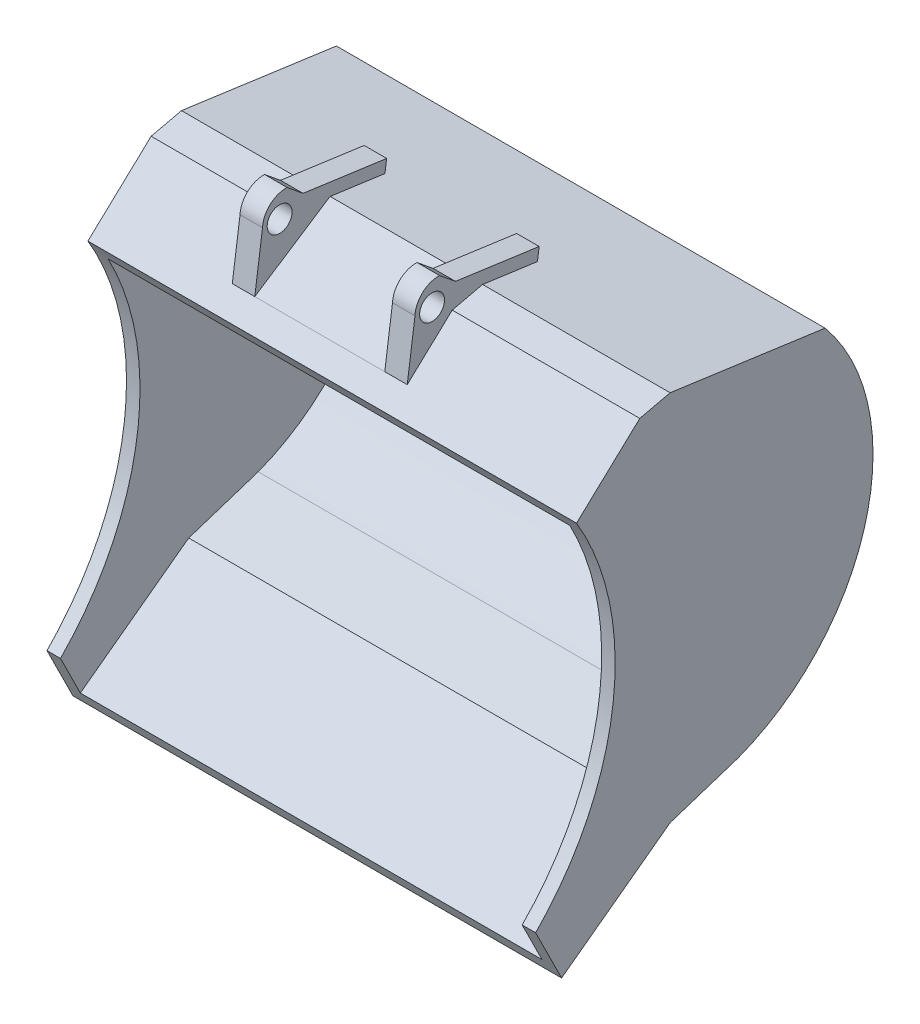
ISO-10303-21;
HEADER;
FILE_DESCRIPTION(('STEP AP214'),'2;1');
FILE_NAME('part.step','',(''),(''),'','','');
FILE_SCHEMA(('AUTOMOTIVE_DESIGN { 1 0 10303 214 1 1 1 1 }'));
ENDSEC;
DATA;
#1=APPLICATION_CONTEXT('core data for automotive mechanical design processes');
#2=APPLICATION_PROTOCOL_DEFINITION('international standard','automotive_design',2000,#1);
#3=PRODUCT_CONTEXT('',#1,'mechanical');
#4=PRODUCT('Part','Part','',(#3));
#5=PRODUCT_RELATED_PRODUCT_CATEGORY('part','',(#4));
#6=PRODUCT_DEFINITION_FORMATION('','',#4);
#7=PRODUCT_DEFINITION_CONTEXT('part definition',#1,'design');
#8=PRODUCT_DEFINITION('design','',#6,#7);
#9=PRODUCT_DEFINITION_SHAPE('','',#8);
#10=(LENGTH_UNIT() NAMED_UNIT(*) SI_UNIT(.MILLI.,.METRE.));
#11=(NAMED_UNIT(*) PLANE_ANGLE_UNIT() SI_UNIT($,.RADIAN.));
#12=(NAMED_UNIT(*) SI_UNIT($,.STERADIAN.) SOLID_ANGLE_UNIT());
#13=UNCERTAINTY_MEASURE_WITH_UNIT(LENGTH_MEASURE(1.E-05),#10,'distance_accuracy_value','');
#14=(GEOMETRIC_REPRESENTATION_CONTEXT(3) GLOBAL_UNCERTAINTY_ASSIGNED_CONTEXT((#13)) GLOBAL_UNIT_ASSIGNED_CONTEXT((#10,
#11,#12)) REPRESENTATION_CONTEXT('',''));
#15=CARTESIAN_POINT('',(0.,0.,0.));
#16=DIRECTION('',(0.,0.,1.));
#17=DIRECTION('',(1.,0.,0.));
#18=AXIS2_PLACEMENT_3D('',#15,#16,#17);
#19=CARTESIAN_POINT('',(1339.,-33.8678557689492,-244.));
#20=DIRECTION('',(0.,0.137484603920545,0.990503903922045));
#21=DIRECTION('',(0.,-0.990503903922045,0.137484603920545));
#22=AXIS2_PLACEMENT_3D('',#19,#20,#21);
#23=PLANE('',#22);
#24=DIRECTION('',(0.,0.990503903922045,-0.137484603920545));
#25=VECTOR('',#24,1.);
#26=CARTESIAN_POINT('',(1239.,-33.8678557689492,-244.));
#27=LINE('',#26,#25);
#28=CARTESIAN_POINT('',(1239.,-33.8678557689492,-244.));
#29=VERTEX_POINT('',#28);
#30=CARTESIAN_POINT('',(1239.,20.6098589467632,-251.56165321563));
#31=VERTEX_POINT('',#30);
#32=EDGE_CURVE('E476',#29,#31,#27,.T.);
#33=ORIENTED_EDGE('',*,*,#32,.T.);
#34=DIRECTION('',(-1.,0.,0.));
#35=VECTOR('',#34,1.);
#36=CARTESIAN_POINT('',(1339.,20.6098589467632,-251.56165321563));
#37=LINE('',#36,#35);
#38=CARTESIAN_POINT('',(1339.,20.6098589467632,-251.56165321563));
#39=VERTEX_POINT('',#38);
#40=EDGE_CURVE('E263',#39,#31,#37,.T.);
#41=ORIENTED_EDGE('',*,*,#40,.F.);
#42=DIRECTION('',(0.,0.990503903922045,-0.137484603920545));
#43=VECTOR('',#42,1.);
#44=CARTESIAN_POINT('',(1339.,-33.8678557689492,-244.));
#45=LINE('',#44,#43);
#46=CARTESIAN_POINT('',(1339.,-33.8678557689492,-244.));
#47=VERTEX_POINT('',#46);
#48=EDGE_CURVE('E501',#47,#39,#45,.T.);
#49=ORIENTED_EDGE('',*,*,#48,.F.);
#50=DIRECTION('',(-1.,0.,0.));
#51=VECTOR('',#50,1.);
#52=CARTESIAN_POINT('',(1339.,-33.8678557689492,-244.));
#53=LINE('',#52,#51);
#54=EDGE_CURVE('E265',#47,#29,#53,.T.);
#55=ORIENTED_EDGE('',*,*,#54,.T.);
#56=EDGE_LOOP('',(#33,#41,#49,#55));
#57=FACE_BOUND('',#56,.T.);
#58=ADVANCED_FACE('F39',(#57),#23,.F.);
#59=CARTESIAN_POINT('',(1339.,20.6098589467632,-251.56165321563));
#60=DIRECTION('',(0.,-0.990503903922045,0.137484603920544));
#61=DIRECTION('',(0.,-0.137484603920544,-0.990503903922045));
#62=AXIS2_PLACEMENT_3D('',#59,#60,#61);
#63=PLANE('',#62);
#64=DIRECTION('',(0.,0.137484603920544,0.990503903922045));
#65=VECTOR('',#64,1.);
#66=CARTESIAN_POINT('',(1239.,20.6098589467632,-251.56165321563));
#67=LINE('',#66,#65);
#68=CARTESIAN_POINT('',(1239.,72.2449516412021,120.441897980372));
#69=VERTEX_POINT('',#68);
#70=EDGE_CURVE('E485',#31,#69,#67,.T.);
#71=ORIENTED_EDGE('',*,*,#70,.T.);
#72=DIRECTION('',(-1.,0.,0.));
#73=VECTOR('',#72,1.);
#74=CARTESIAN_POINT('',(1339.,72.2449516412021,120.441897980372));
#75=LINE('',#74,#73);
#76=CARTESIAN_POINT('',(1339.,72.2449516412021,120.441897980372));
#77=VERTEX_POINT('',#76);
#78=EDGE_CURVE('E443',#77,#69,#75,.T.);
#79=ORIENTED_EDGE('',*,*,#78,.F.);
#80=DIRECTION('',(0.,0.137484603920544,0.990503903922045));
#81=VECTOR('',#80,1.);
#82=CARTESIAN_POINT('',(1339.,20.6098589467632,-251.56165321563));
#83=LINE('',#82,#81);
#84=EDGE_CURVE('E502',#39,#77,#83,.T.);
#85=ORIENTED_EDGE('',*,*,#84,.F.);
#86=ORIENTED_EDGE('',*,*,#40,.T.);
#87=EDGE_LOOP('',(#71,#79,#85,#86));
#88=FACE_BOUND('',#87,.T.);
#89=ADVANCED_FACE('F526',(#88),#63,.F.);
#90=CARTESIAN_POINT('',(1339.,72.2449516412021,120.441897980372));
#91=DIRECTION('',(0.,-0.774121532528882,0.633037007508356));
#92=DIRECTION('',(0.,-0.633037007508356,-0.774121532528882));
#93=AXIS2_PLACEMENT_3D('',#90,#91,#92);
#94=PLANE('',#93);
#95=DIRECTION('',(0.,0.633037007508356,0.774121532528882));
#96=VECTOR('',#95,1.);
#97=CARTESIAN_POINT('',(1239.,72.2449516412021,120.441897980372));
#98=LINE('',#97,#96);
#99=CARTESIAN_POINT('',(1239.,130.129855607766,191.227570914813));
#100=VERTEX_POINT('',#99);
#101=EDGE_CURVE('E484',#69,#100,#98,.T.);
#102=ORIENTED_EDGE('',*,*,#101,.T.);
#103=DIRECTION('',(-1.,0.,0.));
#104=VECTOR('',#103,1.);
#105=CARTESIAN_POINT('',(1339.,130.129855607766,191.227570914813));
#106=LINE('',#105,#104);
#107=CARTESIAN_POINT('',(1339.,130.129855607766,191.227570914813));
#108=VERTEX_POINT('',#107);
#109=EDGE_CURVE('E445',#108,#100,#106,.T.);
#110=ORIENTED_EDGE('',*,*,#109,.F.);
#111=DIRECTION('',(0.,0.633037007508356,0.774121532528882));
#112=VECTOR('',#111,1.);
#113=CARTESIAN_POINT('',(1339.,72.2449516412021,120.441897980372));
#114=LINE('',#113,#112);
#115=EDGE_CURVE('E504',#77,#108,#114,.T.);
#116=ORIENTED_EDGE('',*,*,#115,.F.);
#117=ORIENTED_EDGE('',*,*,#78,.T.);
#118=EDGE_LOOP('',(#102,#110,#116,#117));
#119=FACE_BOUND('',#118,.T.);
#120=ADVANCED_FACE('F529',(#119),#94,.F.);
#121=CARTESIAN_POINT('',(1339.,24.8813249585359,195.369514441472));
#122=DIRECTION('',(-1.,0.,0.));
#123=DIRECTION('',(0.,0.,1.));
#124=AXIS2_PLACEMENT_3D('',#121,#122,#123);
#125=CYLINDRICAL_SURFACE('',#124,105.33);
#126=CARTESIAN_POINT('',(1239.,24.8813249585359,195.369514441472));
#127=DIRECTION('',(1.,0.,0.));
#128=DIRECTION('',(0.,0.,1.));
#129=AXIS2_PLACEMENT_3D('',#126,#127,#128);
#130=CIRCLE('',#129,105.33);
#131=CARTESIAN_POINT('',(1239.,29.4466592998224,300.600529937628));
#132=VERTEX_POINT('',#131);
#133=EDGE_CURVE('E490',#100,#132,#130,.T.);
#134=ORIENTED_EDGE('',*,*,#133,.T.);
#135=DIRECTION('',(-1.,0.,0.));
#136=VECTOR('',#135,1.);
#137=CARTESIAN_POINT('',(1339.,29.4466592998224,300.600529937628));
#138=LINE('',#137,#136);
#139=CARTESIAN_POINT('',(1339.,29.4466592998224,300.600529937628));
#140=VERTEX_POINT('',#139);
#141=EDGE_CURVE('E437',#140,#132,#138,.T.);
#142=ORIENTED_EDGE('',*,*,#141,.F.);
#143=CARTESIAN_POINT('',(1339.,24.8813249585359,195.369514441472));
#144=DIRECTION('',(1.,0.,0.));
#145=DIRECTION('',(0.,0.,1.));
#146=AXIS2_PLACEMENT_3D('',#143,#144,#145);
#147=CIRCLE('',#146,105.33);
#148=EDGE_CURVE('E508',#108,#140,#147,.T.);
#149=ORIENTED_EDGE('',*,*,#148,.F.);
#150=ORIENTED_EDGE('',*,*,#109,.T.);
#151=EDGE_LOOP('',(#134,#142,#149,#150));
#152=FACE_BOUND('',#151,.T.);
#153=ADVANCED_FACE('F535',(#152),#125,.T.);
#154=CARTESIAN_POINT('',(1339.,-218.383340700178,335.));
#155=DIRECTION('',(0.,-0.137484603920545,-0.990503903922045));
#156=DIRECTION('',(0.,0.990503903922045,-0.137484603920545));
#157=AXIS2_PLACEMENT_3D('',#154,#155,#156);
#158=PLANE('',#157);
#159=DIRECTION('',(0.,-0.990503903922044,0.137484603920545));
#160=VECTOR('',#159,1.);
#161=CARTESIAN_POINT('',(1239.,-218.383340700178,335.));
#162=LINE('',#161,#160);
#163=CARTESIAN_POINT('',(1239.,-218.383340700178,335.));
#164=VERTEX_POINT('',#163);
#165=EDGE_CURVE('E489',#132,#164,#162,.T.);
#166=ORIENTED_EDGE('',*,*,#165,.T.);
#167=DIRECTION('',(-1.,0.,0.));
#168=VECTOR('',#167,1.);
#169=CARTESIAN_POINT('',(1339.,-218.383340700178,335.));
#170=LINE('',#169,#168);
#171=CARTESIAN_POINT('',(1339.,-218.383340700178,335.));
#172=VERTEX_POINT('',#171);
#173=EDGE_CURVE('E432',#172,#164,#170,.T.);
#174=ORIENTED_EDGE('',*,*,#173,.F.);
#175=DIRECTION('',(0.,-0.990503903922044,0.137484603920545));
#176=VECTOR('',#175,1.);
#177=CARTESIAN_POINT('',(1339.,-218.383340700178,335.));
#178=LINE('',#177,#176);
#179=EDGE_CURVE('E419',#140,#172,#178,.T.);
#180=ORIENTED_EDGE('',*,*,#179,.F.);
#181=ORIENTED_EDGE('',*,*,#141,.T.);
#182=EDGE_LOOP('',(#166,#174,#180,#181));
#183=FACE_BOUND('',#182,.T.);
#184=ADVANCED_FACE('F513',(#183),#158,.F.);
#185=CARTESIAN_POINT('',(1339.,24.8813249585359,224.465292997617));
#186=DIRECTION('',(-1.,0.,0.));
#187=DIRECTION('',(0.,0.,1.));
#188=AXIS2_PLACEMENT_3D('',#185,#186,#187);
#189=CYLINDRICAL_SURFACE('',#188,55.335);
#190=CARTESIAN_POINT('',(1339.,24.8813249585359,224.465292997617));
#191=DIRECTION('',(1.,0.,0.));
#192=DIRECTION('',(0.,0.,-1.));
#193=AXIS2_PLACEMENT_3D('',#190,#191,#192);
#194=CIRCLE('',#193,55.335);
#195=CARTESIAN_POINT('',(1339.,24.8813249585359,169.130292997617));
#196=VERTEX_POINT('',#195);
#197=EDGE_CURVE('E415',#196,#196,#194,.T.);
#198=ORIENTED_EDGE('',*,*,#197,.T.);
#199=EDGE_LOOP('',(#198));
#200=FACE_BOUND('',#199,.T.);
#201=CARTESIAN_POINT('',(1239.,24.8813249585359,224.465292997617));
#202=DIRECTION('',(1.,0.,0.));
#203=DIRECTION('',(0.,0.,-1.));
#204=AXIS2_PLACEMENT_3D('',#201,#202,#203);
#205=CIRCLE('',#204,55.335);
#206=CARTESIAN_POINT('',(1239.,24.8813249585359,169.130292997617));
#207=VERTEX_POINT('',#206);
#208=EDGE_CURVE('E581',#207,#207,#205,.T.);
#209=ORIENTED_EDGE('',*,*,#208,.F.);
#210=EDGE_LOOP('',(#209));
#211=FACE_BOUND('',#210,.T.);
#212=ADVANCED_FACE('F550',(#200,#211),#189,.F.);
#213=CARTESIAN_POINT('',(2173.,0.,0.));
#214=DIRECTION('',(0.,-0.990503903922045,0.137484603920545));
#215=DIRECTION('',(0.,-0.137484603920545,-0.990503903922045));
#216=AXIS2_PLACEMENT_3D('',#213,#214,#215);
#217=PLANE('',#216);
#218=DIRECTION('',(0.,-0.137484603920545,-0.990503903922045));
#219=VECTOR('',#218,1.);
#220=CARTESIAN_POINT('',(1339.,0.,0.));
#221=LINE('',#220,#219);
#222=CARTESIAN_POINT('',(1339.,0.,0.));
#223=VERTEX_POINT('',#222);
#224=EDGE_CURVE('E433',#223,#47,#221,.T.);
#225=ORIENTED_EDGE('',*,*,#224,.F.);
#226=DIRECTION('',(-1.,0.,0.));
#227=VECTOR('',#226,1.);
#228=CARTESIAN_POINT('',(2173.,0.,0.));
#229=LINE('',#228,#227);
#230=CARTESIAN_POINT('',(2173.,0.,0.));
#231=VERTEX_POINT('',#230);
#232=EDGE_CURVE('E395',#231,#223,#229,.T.);
#233=ORIENTED_EDGE('',*,*,#232,.F.);
#234=DIRECTION('',(0.,0.137484603920545,0.990503903922045));
#235=VECTOR('',#234,1.);
#236=CARTESIAN_POINT('',(2173.,0.,0.));
#237=LINE('',#236,#235);
#238=CARTESIAN_POINT('',(2173.,-95.6350517410083,-689.));
#239=VERTEX_POINT('',#238);
#240=EDGE_CURVE('E334',#239,#231,#237,.T.);
#241=ORIENTED_EDGE('',*,*,#240,.F.);
#242=DIRECTION('',(-1.,0.,0.));
#243=VECTOR('',#242,1.);
#244=CARTESIAN_POINT('',(2173.,-95.6350517410083,-689.));
#245=LINE('',#244,#243);
#246=CARTESIAN_POINT('',(0.,-95.6350517410083,-689.));
#247=VERTEX_POINT('',#246);
#248=EDGE_CURVE('E351',#239,#247,#245,.T.);
#249=ORIENTED_EDGE('',*,*,#248,.T.);
#250=DIRECTION('',(0.,0.137484603920545,0.990503903922045));
#251=VECTOR('',#250,1.);
#252=CARTESIAN_POINT('',(0.,0.,0.));
#253=LINE('',#252,#251);
#254=CARTESIAN_POINT('',(0.,0.,0.));
#255=VERTEX_POINT('',#254);
#256=EDGE_CURVE('E285',#247,#255,#253,.T.);
#257=ORIENTED_EDGE('',*,*,#256,.T.);
#258=CARTESIAN_POINT('',(561.,0.,0.));
#259=VERTEX_POINT('',#258);
#260=EDGE_CURVE('E391',#259,#255,#229,.T.);
#261=ORIENTED_EDGE('',*,*,#260,.F.);
#262=DIRECTION('',(0.,-0.137484603920545,-0.990503903922045));
#263=VECTOR('',#262,1.);
#264=CARTESIAN_POINT('',(561.,0.,0.));
#265=LINE('',#264,#263);
#266=CARTESIAN_POINT('',(561.,-33.8678557689492,-244.));
#267=VERTEX_POINT('',#266);
#268=EDGE_CURVE('E257',#259,#267,#265,.T.);
#269=ORIENTED_EDGE('',*,*,#268,.T.);
#270=CARTESIAN_POINT('',(661.,-33.8678557689492,-244.));
#271=VERTEX_POINT('',#270);
#272=EDGE_CURVE('E65',#271,#267,#53,.T.);
#273=ORIENTED_EDGE('',*,*,#272,.F.);
#274=DIRECTION('',(0.,-0.137484603920545,-0.990503903922045));
#275=VECTOR('',#274,1.);
#276=CARTESIAN_POINT('',(661.,0.,0.));
#277=LINE('',#276,#275);
#278=CARTESIAN_POINT('',(661.,0.,0.));
#279=VERTEX_POINT('',#278);
#280=EDGE_CURVE('E244',#279,#271,#277,.T.);
#281=ORIENTED_EDGE('',*,*,#280,.F.);
#282=DIRECTION('',(1.,0.,0.));
#283=VECTOR('',#282,1.);
#284=CARTESIAN_POINT('',(661.,0.,0.));
#285=LINE('',#284,#283);
#286=CARTESIAN_POINT('',(1239.,0.,0.));
#287=VERTEX_POINT('',#286);
#288=EDGE_CURVE('E493',#279,#287,#285,.T.);
#289=ORIENTED_EDGE('',*,*,#288,.T.);
#290=DIRECTION('',(0.,-0.137484603920545,-0.990503903922045));
#291=VECTOR('',#290,1.);
#292=CARTESIAN_POINT('',(1239.,0.,0.));
#293=LINE('',#292,#291);
#294=EDGE_CURVE('E474',#287,#29,#293,.T.);
#295=ORIENTED_EDGE('',*,*,#294,.T.);
#296=ORIENTED_EDGE('',*,*,#54,.F.);
#297=EDGE_LOOP('',(#225,#233,#241,#249,#257,#261,#269,#273,#281,#289,#295,#296));
#298=FACE_BOUND('',#297,.T.);
#299=ADVANCED_FACE('F41',(#298),#217,.F.);
#300=CARTESIAN_POINT('',(2173.,0.,0.));
#301=DIRECTION('',(0.,-0.974101667469916,-0.226110462898843));
#302=DIRECTION('',(0.,0.226110462898843,-0.974101667469916));
#303=AXIS2_PLACEMENT_3D('',#300,#301,#302);
#304=PLANE('',#303);
#305=DIRECTION('',(0.,0.226110462898843,-0.974101667469916));
#306=VECTOR('',#305,1.);
#307=CARTESIAN_POINT('',(1339.,0.,0.));
#308=LINE('',#307,#306);
#309=CARTESIAN_POINT('',(1339.,-31.3039778545289,134.86));
#310=VERTEX_POINT('',#309);
#311=EDGE_CURVE('E275',#310,#223,#308,.T.);
#312=ORIENTED_EDGE('',*,*,#311,.F.);
#313=DIRECTION('',(-1.,0.,0.));
#314=VECTOR('',#313,1.);
#315=CARTESIAN_POINT('',(2173.,-31.3039778545289,134.86));
#316=LINE('',#315,#314);
#317=CARTESIAN_POINT('',(2173.,-31.3039778545289,134.86));
#318=VERTEX_POINT('',#317);
#319=EDGE_CURVE('E389',#318,#310,#316,.T.);
#320=ORIENTED_EDGE('',*,*,#319,.F.);
#321=DIRECTION('',(0.,-0.226110462898843,0.974101667469916));
#322=VECTOR('',#321,1.);
#323=CARTESIAN_POINT('',(2173.,0.,0.));
#324=LINE('',#323,#322);
#325=EDGE_CURVE('E336',#231,#318,#324,.T.);
#326=ORIENTED_EDGE('',*,*,#325,.F.);
#327=ORIENTED_EDGE('',*,*,#232,.T.);
#328=EDGE_LOOP('',(#312,#320,#326,#327));
#329=FACE_BOUND('',#328,.T.);
#330=ADVANCED_FACE('F519',(#329),#304,.F.);
#331=CARTESIAN_POINT('',(2173.,-31.3039778545289,134.86));
#332=DIRECTION('',(0.,-0.730541558448307,-0.682868238666816));
#333=DIRECTION('',(0.,0.682868238666816,-0.730541558448307));
#334=AXIS2_PLACEMENT_3D('',#331,#332,#333);
#335=PLANE('',#334);
#336=DIRECTION('',(0.,0.682868238666816,-0.730541558448307));
#337=VECTOR('',#336,1.);
#338=CARTESIAN_POINT('',(1339.,-31.3039778545289,134.86));
#339=LINE('',#338,#337);
#340=EDGE_CURVE('E11',#172,#310,#339,.T.);
#341=ORIENTED_EDGE('',*,*,#340,.F.);
#342=ORIENTED_EDGE('',*,*,#173,.T.);
#343=DIRECTION('',(1.,0.,0.));
#344=VECTOR('',#343,1.);
#345=CARTESIAN_POINT('',(661.,-218.383340700178,335.));
#346=LINE('',#345,#344);
#347=CARTESIAN_POINT('',(661.,-218.383340700178,335.));
#348=VERTEX_POINT('',#347);
#349=EDGE_CURVE('E475',#348,#164,#346,.T.);
#350=ORIENTED_EDGE('',*,*,#349,.F.);
#351=CARTESIAN_POINT('',(561.,-218.383340700178,335.));
#352=VERTEX_POINT('',#351);
#353=EDGE_CURVE('E399',#348,#352,#170,.T.);
#354=ORIENTED_EDGE('',*,*,#353,.T.);
#355=DIRECTION('',(0.,0.682868238666816,-0.730541558448307));
#356=VECTOR('',#355,1.);
#357=CARTESIAN_POINT('',(561.,-31.3039778545289,134.86));
#358=LINE('',#357,#356);
#359=CARTESIAN_POINT('',(561.,-31.3039778545289,134.86));
#360=VERTEX_POINT('',#359);
#361=EDGE_CURVE('E50',#352,#360,#358,.T.);
#362=ORIENTED_EDGE('',*,*,#361,.T.);
#363=CARTESIAN_POINT('',(0.,-31.3039778545289,134.86));
#364=VERTEX_POINT('',#363);
#365=EDGE_CURVE('E390',#360,#364,#316,.T.);
#366=ORIENTED_EDGE('',*,*,#365,.T.);
#367=DIRECTION('',(0.,-0.682868238666816,0.730541558448307));
#368=VECTOR('',#367,1.);
#369=CARTESIAN_POINT('',(0.,-31.3039778545289,134.86));
#370=LINE('',#369,#368);
#371=CARTESIAN_POINT('',(0.,-294.208249741253,416.118500002598));
#372=VERTEX_POINT('',#371);
#373=EDGE_CURVE('E360',#364,#372,#370,.T.);
#374=ORIENTED_EDGE('',*,*,#373,.T.);
#375=DIRECTION('',(-1.,0.,0.));
#376=VECTOR('',#375,1.);
#377=CARTESIAN_POINT('',(2173.,-294.208249741253,416.118500002598));
#378=LINE('',#377,#376);
#379=CARTESIAN_POINT('',(2173.,-294.208249741253,416.118500002598));
#380=VERTEX_POINT('',#379);
#381=EDGE_CURVE('E383',#380,#372,#378,.T.);
#382=ORIENTED_EDGE('',*,*,#381,.F.);
#383=DIRECTION('',(0.,-0.682868238666816,0.730541558448307));
#384=VECTOR('',#383,1.);
#385=CARTESIAN_POINT('',(2173.,-31.3039778545289,134.86));
#386=LINE('',#385,#384);
#387=EDGE_CURVE('E338',#318,#380,#386,.T.);
#388=ORIENTED_EDGE('',*,*,#387,.F.);
#389=ORIENTED_EDGE('',*,*,#319,.T.);
#390=EDGE_LOOP('',(#341,#342,#350,#354,#362,#366,#374,#382,#388,#389));
#391=FACE_BOUND('',#390,.T.);
#392=ADVANCED_FACE('F400',(#391),#335,.F.);
#393=CARTESIAN_POINT('',(2173.,-919.634284323021,1469.4310249767));
#394=DIRECTION('',(-1.,0.,0.));
#395=DIRECTION('',(0.,0.,1.));
#396=AXIS2_PLACEMENT_3D('',#393,#394,#395);
#397=CYLINDRICAL_SURFACE('',#396,1225.);
#398=CARTESIAN_POINT('',(60.0000000000001,-919.634284323021,1469.4310249767));
#399=DIRECTION('',(-1.,0.,0.));
#400=DIRECTION('',(0.,0.,1.));
#401=AXIS2_PLACEMENT_3D('',#398,#399,#400);
#402=CIRCLE('',#401,1225.);
#403=CARTESIAN_POINT('',(60.,-348.114078031214,385.922993718895));
#404=VERTEX_POINT('',#403);
#405=CARTESIAN_POINT('',(60.0000000000001,-1780.60824974125,598.02478740894));
#406=VERTEX_POINT('',#405);
#407=EDGE_CURVE('E305',#404,#406,#402,.T.);
#408=ORIENTED_EDGE('',*,*,#407,.F.);
#409=DIRECTION('',(-1.,0.,0.));
#410=VECTOR('',#409,1.);
#411=CARTESIAN_POINT('',(2113.,-348.114078031214,385.922993718895));
#412=LINE('',#411,#410);
#413=CARTESIAN_POINT('',(2113.,-348.114078031214,385.922993718895));
#414=VERTEX_POINT('',#413);
#415=EDGE_CURVE('E297',#414,#404,#412,.T.);
#416=ORIENTED_EDGE('',*,*,#415,.F.);
#417=CARTESIAN_POINT('',(2113.,-919.634284323021,1469.4310249767));
#418=DIRECTION('',(-1.,0.,0.));
#419=DIRECTION('',(0.,0.,1.));
#420=AXIS2_PLACEMENT_3D('',#417,#418,#419);
#421=CIRCLE('',#420,1225.);
#422=CARTESIAN_POINT('',(2113.,-1780.60824974125,598.02478740894));
#423=VERTEX_POINT('',#422);
#424=EDGE_CURVE('E302',#414,#423,#421,.T.);
#425=ORIENTED_EDGE('',*,*,#424,.T.);
#426=DIRECTION('',(-1.,0.,0.));
#427=VECTOR('',#426,1.);
#428=CARTESIAN_POINT('',(2173.,-1780.60824974125,598.02478740894));
#429=LINE('',#428,#427);
#430=CARTESIAN_POINT('',(2173.,-1780.60824974125,598.02478740894));
#431=VERTEX_POINT('',#430);
#432=EDGE_CURVE('E381',#431,#423,#429,.T.);
#433=ORIENTED_EDGE('',*,*,#432,.F.);
#434=CARTESIAN_POINT('',(2173.,-919.634284323021,1469.4310249767));
#435=DIRECTION('',(-1.,0.,0.));
#436=DIRECTION('',(0.,0.,1.));
#437=AXIS2_PLACEMENT_3D('',#434,#435,#436);
#438=CIRCLE('',#437,1225.);
#439=EDGE_CURVE('E343',#380,#431,#438,.T.);
#440=ORIENTED_EDGE('',*,*,#439,.F.);
#441=ORIENTED_EDGE('',*,*,#381,.T.);
#442=CARTESIAN_POINT('',(0.,-919.634284323021,1469.4310249767));
#443=DIRECTION('',(-1.,0.,0.));
#444=DIRECTION('',(0.,0.,1.));
#445=AXIS2_PLACEMENT_3D('',#442,#443,#444);
#446=CIRCLE('',#445,1225.);
#447=CARTESIAN_POINT('',(0.,-1780.60824974125,598.02478740894));
#448=VERTEX_POINT('',#447);
#449=EDGE_CURVE('E357',#372,#448,#446,.T.);
#450=ORIENTED_EDGE('',*,*,#449,.T.);
#451=EDGE_CURVE('E379',#406,#448,#429,.T.);
#452=ORIENTED_EDGE('',*,*,#451,.F.);
#453=EDGE_LOOP('',(#408,#416,#425,#433,#440,#441,#450,#452));
#454=FACE_BOUND('',#453,.T.);
#455=ADVANCED_FACE('F605',(#454),#397,.F.);
#456=CARTESIAN_POINT('',(2173.,-2012.60824974125,482.525187131697));
#457=DIRECTION('',(0.,0.445668249515807,-0.895198196699209));
#458=DIRECTION('',(0.,0.895198196699209,0.445668249515807));
#459=AXIS2_PLACEMENT_3D('',#456,#457,#458);
#460=PLANE('',#459);
#461=DIRECTION('',(0.,-0.895198196699209,-0.445668249515807));
#462=VECTOR('',#461,1.);
#463=CARTESIAN_POINT('',(60.,-1132.73844899319,920.562300417985));
#464=LINE('',#463,#462);
#465=CARTESIAN_POINT('',(60.,-1958.06776543082,509.67779116955));
#466=VERTEX_POINT('',#465);
#467=EDGE_CURVE('E314',#406,#466,#464,.T.);
#468=ORIENTED_EDGE('',*,*,#467,.F.);
#469=ORIENTED_EDGE('',*,*,#451,.T.);
#470=DIRECTION('',(0.,-0.895198196699209,-0.445668249515807));
#471=VECTOR('',#470,1.);
#472=CARTESIAN_POINT('',(0.,-2012.60824974125,482.525187131697));
#473=LINE('',#472,#471);
#474=CARTESIAN_POINT('',(0.,-2012.60824974125,482.525187131697));
#475=VERTEX_POINT('',#474);
#476=EDGE_CURVE('E362',#448,#475,#473,.T.);
#477=ORIENTED_EDGE('',*,*,#476,.T.);
#478=DIRECTION('',(-1.,0.,0.));
#479=VECTOR('',#478,1.);
#480=CARTESIAN_POINT('',(2173.,-2012.60824974125,482.525187131697));
#481=LINE('',#480,#479);
#482=CARTESIAN_POINT('',(2173.,-2012.60824974125,482.525187131697));
#483=VERTEX_POINT('',#482);
#484=EDGE_CURVE('E380',#483,#475,#481,.T.);
#485=ORIENTED_EDGE('',*,*,#484,.F.);
#486=DIRECTION('',(0.,-0.895198196699209,-0.445668249515807));
#487=VECTOR('',#486,1.);
#488=CARTESIAN_POINT('',(2173.,-2012.60824974125,482.525187131697));
#489=LINE('',#488,#487);
#490=EDGE_CURVE('E341',#431,#483,#489,.T.);
#491=ORIENTED_EDGE('',*,*,#490,.F.);
#492=ORIENTED_EDGE('',*,*,#432,.T.);
#493=DIRECTION('',(0.,-0.895198196699209,-0.445668249515807));
#494=VECTOR('',#493,1.);
#495=CARTESIAN_POINT('',(2113.,-1132.73844899319,920.562300417985));
#496=LINE('',#495,#494);
#497=CARTESIAN_POINT('',(2113.,-1958.06776543082,509.67779116955));
#498=VERTEX_POINT('',#497);
#499=EDGE_CURVE('E306',#423,#498,#496,.T.);
#500=ORIENTED_EDGE('',*,*,#499,.T.);
#501=DIRECTION('',(-1.,0.,0.));
#502=VECTOR('',#501,1.);
#503=CARTESIAN_POINT('',(2173.,-1958.06776543082,509.67779116955));
#504=LINE('',#503,#502);
#505=EDGE_CURVE('E318',#498,#466,#504,.T.);
#506=ORIENTED_EDGE('',*,*,#505,.T.);
#507=EDGE_LOOP('',(#468,#469,#477,#485,#491,#492,#500,#506));
#508=FACE_BOUND('',#507,.T.);
#509=ADVANCED_FACE('F604',(#508),#460,.F.);
#510=ORIENTED_EDGE('',*,*,#365,.F.);
#511=DIRECTION('',(0.,0.226110462898843,-0.974101667469916));
#512=VECTOR('',#511,1.);
#513=CARTESIAN_POINT('',(561.,0.,0.));
#514=LINE('',#513,#512);
#515=EDGE_CURVE('E266',#360,#259,#514,.T.);
#516=ORIENTED_EDGE('',*,*,#515,.T.);
#517=ORIENTED_EDGE('',*,*,#260,.T.);
#518=DIRECTION('',(0.,-0.226110462898843,0.974101667469916));
#519=VECTOR('',#518,1.);
#520=CARTESIAN_POINT('',(0.,0.,0.));
#521=LINE('',#520,#519);
#522=EDGE_CURVE('E353',#255,#364,#521,.T.);
#523=ORIENTED_EDGE('',*,*,#522,.T.);
#524=EDGE_LOOP('',(#510,#516,#517,#523));
#525=FACE_BOUND('',#524,.T.);
#526=ADVANCED_FACE('F406',(#525),#304,.F.);
#527=CARTESIAN_POINT('',(2173.,-1656.,-2.02801509938802E-13));
#528=DIRECTION('',(0.,0.804208645219496,0.59434708290209));
#529=DIRECTION('',(0.,-0.59434708290209,0.804208645219496));
#530=AXIS2_PLACEMENT_3D('',#527,#528,#529);
#531=PLANE('',#530);
#532=DIRECTION('',(0.,0.59434708290209,-0.804208645219496));
#533=VECTOR('',#532,1.);
#534=CARTESIAN_POINT('',(0.,-1656.,-2.02801509938802E-13));
#535=LINE('',#534,#533);
#536=CARTESIAN_POINT('',(0.,-1656.,-2.02801509938802E-13));
#537=VERTEX_POINT('',#536);
#538=EDGE_CURVE('E365',#475,#537,#535,.T.);
#539=ORIENTED_EDGE('',*,*,#538,.T.);
#540=DIRECTION('',(-1.,0.,0.));
#541=VECTOR('',#540,1.);
#542=CARTESIAN_POINT('',(2173.,-1656.,-2.02801509938802E-13));
#543=LINE('',#542,#541);
#544=CARTESIAN_POINT('',(2173.,-1656.,-2.02801509938802E-13));
#545=VERTEX_POINT('',#544);
#546=EDGE_CURVE('E372',#545,#537,#543,.T.);
#547=ORIENTED_EDGE('',*,*,#546,.F.);
#548=DIRECTION('',(0.,0.59434708290209,-0.804208645219496));
#549=VECTOR('',#548,1.);
#550=CARTESIAN_POINT('',(2173.,-1656.,-2.02801509938802E-13));
#551=LINE('',#550,#549);
#552=EDGE_CURVE('E344',#483,#545,#551,.T.);
#553=ORIENTED_EDGE('',*,*,#552,.F.);
#554=ORIENTED_EDGE('',*,*,#484,.T.);
#555=EDGE_LOOP('',(#539,#547,#553,#554));
#556=FACE_BOUND('',#555,.T.);
#557=ADVANCED_FACE('F603',(#556),#531,.F.);
#558=CARTESIAN_POINT('',(2173.,-1656.,-2.02801509938802E-13));
#559=DIRECTION('',(0.,0.951056516295152,0.309016994374952));
#560=DIRECTION('',(0.,-0.309016994374952,0.951056516295152));
#561=AXIS2_PLACEMENT_3D('',#558,#559,#560);
#562=PLANE('',#561);
#563=DIRECTION('',(0.,0.309016994374952,-0.951056516295152));
#564=VECTOR('',#563,1.);
#565=CARTESIAN_POINT('',(0.,-1656.,-2.02801509938802E-13));
#566=LINE('',#565,#564);
#567=CARTESIAN_POINT('',(0.,-1558.12025642121,-301.242875435373));
#568=VERTEX_POINT('',#567);
#569=EDGE_CURVE('E368',#537,#568,#566,.T.);
#570=ORIENTED_EDGE('',*,*,#569,.T.);
#571=DIRECTION('',(-1.,0.,0.));
#572=VECTOR('',#571,1.);
#573=CARTESIAN_POINT('',(2173.,-1558.12025642121,-301.242875435373));
#574=LINE('',#573,#572);
#575=CARTESIAN_POINT('',(2173.,-1558.12025642121,-301.242875435373));
#576=VERTEX_POINT('',#575);
#577=EDGE_CURVE('E371',#576,#568,#574,.T.);
#578=ORIENTED_EDGE('',*,*,#577,.F.);
#579=DIRECTION('',(0.,0.309016994374952,-0.951056516295152));
#580=VECTOR('',#579,1.);
#581=CARTESIAN_POINT('',(2173.,-1656.,-2.02801509938802E-13));
#582=LINE('',#581,#580);
#583=EDGE_CURVE('E350',#545,#576,#582,.T.);
#584=ORIENTED_EDGE('',*,*,#583,.F.);
#585=ORIENTED_EDGE('',*,*,#546,.T.);
#586=EDGE_LOOP('',(#570,#578,#584,#585));
#587=FACE_BOUND('',#586,.T.);
#588=ADVANCED_FACE('F606',(#587),#562,.F.);
#589=CARTESIAN_POINT('',(2173.,-688.25,27.7339276886459));
#590=DIRECTION('',(-1.,0.,0.));
#591=DIRECTION('',(0.,0.,1.));
#592=AXIS2_PLACEMENT_3D('',#589,#590,#591);
#593=CYLINDRICAL_SURFACE('',#592,930.);
#594=CARTESIAN_POINT('',(0.,-688.25,27.7339276886459));
#595=DIRECTION('',(1.,0.,0.));
#596=DIRECTION('',(0.,0.,1.));
#597=AXIS2_PLACEMENT_3D('',#594,#595,#596);
#598=CIRCLE('',#597,930.);
#599=EDGE_CURVE('E340',#568,#247,#598,.T.);
#600=ORIENTED_EDGE('',*,*,#599,.T.);
#601=ORIENTED_EDGE('',*,*,#248,.F.);
#602=CARTESIAN_POINT('',(2173.,-688.25,27.7339276886459));
#603=DIRECTION('',(1.,0.,0.));
#604=DIRECTION('',(0.,0.,1.));
#605=AXIS2_PLACEMENT_3D('',#602,#603,#604);
#606=CIRCLE('',#605,930.);
#607=EDGE_CURVE('E349',#576,#239,#606,.T.);
#608=ORIENTED_EDGE('',*,*,#607,.F.);
#609=ORIENTED_EDGE('',*,*,#577,.T.);
#610=EDGE_LOOP('',(#600,#601,#608,#609));
#611=FACE_BOUND('',#610,.T.);
#612=ADVANCED_FACE('F623',(#611),#593,.T.);
#613=CARTESIAN_POINT('',(2173.,-688.25,27.7339276886459));
#614=DIRECTION('',(-1.,0.,0.));
#615=DIRECTION('',(0.,0.,1.));
#616=AXIS2_PLACEMENT_3D('',#613,#614,#615);
#617=PLANE('',#616);
#618=ORIENTED_EDGE('',*,*,#240,.T.);
#619=ORIENTED_EDGE('',*,*,#325,.T.);
#620=ORIENTED_EDGE('',*,*,#387,.T.);
#621=ORIENTED_EDGE('',*,*,#439,.T.);
#622=ORIENTED_EDGE('',*,*,#490,.T.);
#623=ORIENTED_EDGE('',*,*,#552,.T.);
#624=ORIENTED_EDGE('',*,*,#583,.T.);
#625=ORIENTED_EDGE('',*,*,#607,.T.);
#626=EDGE_LOOP('',(#618,#619,#620,#621,#622,#623,#624,#625));
#627=FACE_BOUND('',#626,.T.);
#628=ADVANCED_FACE('F628',(#627),#617,.F.);
#629=CARTESIAN_POINT('',(0.,-688.25,27.7339276886459));
#630=DIRECTION('',(-1.,0.,0.));
#631=DIRECTION('',(0.,0.,1.));
#632=AXIS2_PLACEMENT_3D('',#629,#630,#631);
#633=PLANE('',#632);
#634=ORIENTED_EDGE('',*,*,#256,.F.);
#635=ORIENTED_EDGE('',*,*,#599,.F.);
#636=ORIENTED_EDGE('',*,*,#569,.F.);
#637=ORIENTED_EDGE('',*,*,#538,.F.);
#638=ORIENTED_EDGE('',*,*,#476,.F.);
#639=ORIENTED_EDGE('',*,*,#449,.F.);
#640=ORIENTED_EDGE('',*,*,#373,.F.);
#641=ORIENTED_EDGE('',*,*,#522,.F.);
#642=EDGE_LOOP('',(#634,#635,#636,#637,#638,#639,#640,#641));
#643=FACE_BOUND('',#642,.T.);
#644=ADVANCED_FACE('F633',(#643),#633,.T.);
#645=CARTESIAN_POINT('',(2173.,-59.4302342353227,8.24907623523268));
#646=DIRECTION('',(0.,-0.990503903922045,0.137484603920545));
#647=DIRECTION('',(0.,-0.137484603920545,-0.990503903922045));
#648=AXIS2_PLACEMENT_3D('',#645,#646,#647);
#649=PLANE('',#648);
#650=DIRECTION('',(0.,0.137484603920545,0.990503903922045));
#651=VECTOR('',#650,1.);
#652=CARTESIAN_POINT('',(60.,-68.6627674018115,-58.2664453847878));
#653=LINE('',#652,#651);
#654=CARTESIAN_POINT('',(60.,-151.794421903552,-657.186076931753));
#655=VERTEX_POINT('',#654);
#656=CARTESIAN_POINT('',(60.,-60.9569139254462,-2.74984400735522));
#657=VERTEX_POINT('',#656);
#658=EDGE_CURVE('E274',#655,#657,#653,.T.);
#659=ORIENTED_EDGE('',*,*,#658,.F.);
#660=DIRECTION('',(-1.,0.,0.));
#661=VECTOR('',#660,1.);
#662=CARTESIAN_POINT('',(2113.,-151.794421903552,-657.186076931753));
#663=LINE('',#662,#661);
#664=CARTESIAN_POINT('',(2113.,-151.794421903552,-657.186076931753));
#665=VERTEX_POINT('',#664);
#666=EDGE_CURVE('E287',#665,#655,#663,.T.);
#667=ORIENTED_EDGE('',*,*,#666,.F.);
#668=DIRECTION('',(0.,0.137484603920545,0.990503903922045));
#669=VECTOR('',#668,1.);
#670=CARTESIAN_POINT('',(2113.,-68.6627674018115,-58.2664453847878));
#671=LINE('',#670,#669);
#672=CARTESIAN_POINT('',(2113.,-60.9569139254462,-2.74984400735522));
#673=VERTEX_POINT('',#672);
#674=EDGE_CURVE('E283',#665,#673,#671,.T.);
#675=ORIENTED_EDGE('',*,*,#674,.T.);
#676=DIRECTION('',(-1.,0.,0.));
#677=VECTOR('',#676,1.);
#678=CARTESIAN_POINT('',(2173.,-60.9569139254462,-2.74984400735522));
#679=LINE('',#678,#677);
#680=EDGE_CURVE('E276',#673,#657,#679,.T.);
#681=ORIENTED_EDGE('',*,*,#680,.T.);
#682=EDGE_LOOP('',(#659,#667,#675,#681));
#683=FACE_BOUND('',#682,.T.);
#684=ADVANCED_FACE('F632',(#683),#649,.T.);
#685=CARTESIAN_POINT('',(2173.,-58.446100048195,-13.5666277739306));
#686=DIRECTION('',(0.,-0.974101667469916,-0.226110462898843));
#687=DIRECTION('',(0.,0.226110462898843,-0.974101667469916));
#688=AXIS2_PLACEMENT_3D('',#685,#686,#687);
#689=PLANE('',#688);
#690=DIRECTION('',(0.,-0.226110462898843,0.974101667469916));
#691=VECTOR('',#690,1.);
#692=CARTESIAN_POINT('',(60.,-99.7420538044702,164.339590708957));
#693=LINE('',#692,#691);
#694=CARTESIAN_POINT('',(60.,-86.1149109466855,105.632786917407));
#695=VERTEX_POINT('',#694);
#696=EDGE_CURVE('E279',#657,#695,#693,.T.);
#697=ORIENTED_EDGE('',*,*,#696,.F.);
#698=ORIENTED_EDGE('',*,*,#680,.F.);
#699=DIRECTION('',(0.,-0.226110462898843,0.974101667469916));
#700=VECTOR('',#699,1.);
#701=CARTESIAN_POINT('',(2113.,-99.7420538044702,164.339590708957));
#702=LINE('',#701,#700);
#703=CARTESIAN_POINT('',(2113.,-86.1149109466855,105.632786917407));
#704=VERTEX_POINT('',#703);
#705=EDGE_CURVE('E290',#673,#704,#702,.T.);
#706=ORIENTED_EDGE('',*,*,#705,.T.);
#707=DIRECTION('',(-1.,0.,0.));
#708=VECTOR('',#707,1.);
#709=CARTESIAN_POINT('',(2173.,-86.1149109466855,105.632786917407));
#710=LINE('',#709,#708);
#711=EDGE_CURVE('E282',#704,#695,#710,.T.);
#712=ORIENTED_EDGE('',*,*,#711,.T.);
#713=EDGE_LOOP('',(#697,#698,#706,#712));
#714=FACE_BOUND('',#713,.T.);
#715=ADVANCED_FACE('F659',(#714),#689,.T.);
#716=CARTESIAN_POINT('',(2173.,-75.1364713614273,93.8879056799911));
#717=DIRECTION('',(0.,-0.730541558448307,-0.682868238666816));
#718=DIRECTION('',(0.,0.682868238666816,-0.730541558448307));
#719=AXIS2_PLACEMENT_3D('',#716,#717,#718);
#720=PLANE('',#719);
#721=DIRECTION('',(0.,-0.682868238666816,0.730541558448307));
#722=VECTOR('',#721,1.);
#723=CARTESIAN_POINT('',(60.,-328.035033606346,364.442163925238));
#724=LINE('',#723,#722);
#725=EDGE_CURVE('E293',#695,#404,#724,.T.);
#726=ORIENTED_EDGE('',*,*,#725,.F.);
#727=ORIENTED_EDGE('',*,*,#711,.F.);
#728=DIRECTION('',(0.,-0.682868238666816,0.730541558448307));
#729=VECTOR('',#728,1.);
#730=CARTESIAN_POINT('',(2113.,-328.035033606346,364.442163925238));
#731=LINE('',#730,#729);
#732=EDGE_CURVE('E299',#704,#414,#731,.T.);
#733=ORIENTED_EDGE('',*,*,#732,.T.);
#734=ORIENTED_EDGE('',*,*,#415,.T.);
#735=EDGE_LOOP('',(#726,#727,#733,#734));
#736=FACE_BOUND('',#735,.T.);
#737=ADVANCED_FACE('F656',(#736),#720,.T.);
#738=CARTESIAN_POINT('',(2173.,-1607.74748128683,35.6608249741252));
#739=DIRECTION('',(0.,0.804208645219496,0.59434708290209));
#740=DIRECTION('',(0.,-0.59434708290209,0.804208645219496));
#741=AXIS2_PLACEMENT_3D('',#738,#739,#740);
#742=PLANE('',#741);
#743=DIRECTION('',(0.,0.59434708290209,-0.804208645219496));
#744=VECTOR('',#743,1.);
#745=CARTESIAN_POINT('',(60.,-1279.14752575625,-408.966452013734));
#746=LINE('',#745,#744);
#747=CARTESIAN_POINT('',(60.,-1601.95057574235,27.8170554184155));
#748=VERTEX_POINT('',#747);
#749=EDGE_CURVE('E313',#466,#748,#746,.T.);
#750=ORIENTED_EDGE('',*,*,#749,.F.);
#751=ORIENTED_EDGE('',*,*,#505,.F.);
#752=DIRECTION('',(0.,0.59434708290209,-0.804208645219496));
#753=VECTOR('',#752,1.);
#754=CARTESIAN_POINT('',(2113.,-1279.14752575625,-408.966452013734));
#755=LINE('',#754,#753);
#756=CARTESIAN_POINT('',(2113.,-1601.95057574235,27.8170554184155));
#757=VERTEX_POINT('',#756);
#758=EDGE_CURVE('E304',#498,#757,#755,.T.);
#759=ORIENTED_EDGE('',*,*,#758,.T.);
#760=DIRECTION('',(-1.,0.,0.));
#761=VECTOR('',#760,1.);
#762=CARTESIAN_POINT('',(2173.,-1601.95057574235,27.8170554184155));
#763=LINE('',#762,#761);
#764=EDGE_CURVE('E312',#757,#748,#763,.T.);
#765=ORIENTED_EDGE('',*,*,#764,.T.);
#766=EDGE_LOOP('',(#750,#751,#759,#765));
#767=FACE_BOUND('',#766,.T.);
#768=ADVANCED_FACE('F655',(#767),#742,.T.);
#769=CARTESIAN_POINT('',(2173.,-1598.93660902229,18.5410196624969));
#770=DIRECTION('',(0.,0.951056516295152,0.309016994374952));
#771=DIRECTION('',(0.,-0.309016994374952,0.951056516295152));
#772=AXIS2_PLACEMENT_3D('',#769,#770,#771);
#773=PLANE('',#772);
#774=DIRECTION('',(0.,0.309016994374952,-0.951056516295152));
#775=VECTOR('',#774,1.);
#776=CARTESIAN_POINT('',(60.,-1514.67550401723,-240.787996035764));
#777=LINE('',#776,#775);
#778=CARTESIAN_POINT('',(60.,-1501.50375553248,-281.326469503095));
#779=VERTEX_POINT('',#778);
#780=EDGE_CURVE('E311',#748,#779,#777,.T.);
#781=ORIENTED_EDGE('',*,*,#780,.F.);
#782=ORIENTED_EDGE('',*,*,#764,.F.);
#783=DIRECTION('',(0.,0.309016994374952,-0.951056516295152));
#784=VECTOR('',#783,1.);
#785=CARTESIAN_POINT('',(2113.,-1514.67550401723,-240.787996035764));
#786=LINE('',#785,#784);
#787=CARTESIAN_POINT('',(2113.,-1501.50375553248,-281.326469503095));
#788=VERTEX_POINT('',#787);
#789=EDGE_CURVE('E307',#757,#788,#786,.T.);
#790=ORIENTED_EDGE('',*,*,#789,.T.);
#791=DIRECTION('',(-1.,0.,0.));
#792=VECTOR('',#791,1.);
#793=CARTESIAN_POINT('',(2113.,-1501.50375553248,-281.326469503095));
#794=LINE('',#793,#792);
#795=EDGE_CURVE('E295',#788,#779,#794,.T.);
#796=ORIENTED_EDGE('',*,*,#795,.T.);
#797=EDGE_LOOP('',(#781,#782,#790,#796));
#798=FACE_BOUND('',#797,.T.);
#799=ADVANCED_FACE('F648',(#798),#773,.T.);
#800=CARTESIAN_POINT('',(2173.,-688.25,27.7339276886459));
#801=DIRECTION('',(-1.,0.,0.));
#802=DIRECTION('',(0.,0.,1.));
#803=AXIS2_PLACEMENT_3D('',#800,#801,#802);
#804=CYLINDRICAL_SURFACE('',#803,870.);
#805=CARTESIAN_POINT('',(60.0000000000001,-688.25,27.7339276886459));
#806=DIRECTION('',(-1.,0.,0.));
#807=DIRECTION('',(0.,0.,1.));
#808=AXIS2_PLACEMENT_3D('',#805,#806,#807);
#809=CIRCLE('',#808,870.);
#810=EDGE_CURVE('E286',#779,#655,#809,.F.);
#811=ORIENTED_EDGE('',*,*,#810,.F.);
#812=ORIENTED_EDGE('',*,*,#795,.F.);
#813=CARTESIAN_POINT('',(2113.,-688.25,27.7339276886459));
#814=DIRECTION('',(-1.,0.,0.));
#815=DIRECTION('',(0.,0.,1.));
#816=AXIS2_PLACEMENT_3D('',#813,#814,#815);
#817=CIRCLE('',#816,870.);
#818=EDGE_CURVE('E291',#788,#665,#817,.F.);
#819=ORIENTED_EDGE('',*,*,#818,.T.);
#820=ORIENTED_EDGE('',*,*,#666,.T.);
#821=EDGE_LOOP('',(#811,#812,#819,#820));
#822=FACE_BOUND('',#821,.T.);
#823=ADVANCED_FACE('F644',(#822),#804,.F.);
#824=CARTESIAN_POINT('',(2113.,-688.25,27.7339276886459));
#825=DIRECTION('',(-1.,0.,0.));
#826=DIRECTION('',(0.,0.,1.));
#827=AXIS2_PLACEMENT_3D('',#824,#825,#826);
#828=PLANE('',#827);
#829=ORIENTED_EDGE('',*,*,#674,.F.);
#830=ORIENTED_EDGE('',*,*,#818,.F.);
#831=ORIENTED_EDGE('',*,*,#789,.F.);
#832=ORIENTED_EDGE('',*,*,#758,.F.);
#833=ORIENTED_EDGE('',*,*,#499,.F.);
#834=ORIENTED_EDGE('',*,*,#424,.F.);
#835=ORIENTED_EDGE('',*,*,#732,.F.);
#836=ORIENTED_EDGE('',*,*,#705,.F.);
#837=EDGE_LOOP('',(#829,#830,#831,#832,#833,#834,#835,#836));
#838=FACE_BOUND('',#837,.T.);
#839=ADVANCED_FACE('F639',(#838),#828,.T.);
#840=CARTESIAN_POINT('',(60.,-688.25,27.7339276886459));
#841=DIRECTION('',(-1.,0.,0.));
#842=DIRECTION('',(0.,0.,1.));
#843=AXIS2_PLACEMENT_3D('',#840,#841,#842);
#844=PLANE('',#843);
#845=ORIENTED_EDGE('',*,*,#658,.T.);
#846=ORIENTED_EDGE('',*,*,#696,.T.);
#847=ORIENTED_EDGE('',*,*,#725,.T.);
#848=ORIENTED_EDGE('',*,*,#407,.T.);
#849=ORIENTED_EDGE('',*,*,#467,.T.);
#850=ORIENTED_EDGE('',*,*,#749,.T.);
#851=ORIENTED_EDGE('',*,*,#780,.T.);
#852=ORIENTED_EDGE('',*,*,#810,.T.);
#853=EDGE_LOOP('',(#845,#846,#847,#848,#849,#850,#851,#852));
#854=FACE_BOUND('',#853,.T.);
#855=ADVANCED_FACE('F566',(#854),#844,.F.);
#856=CARTESIAN_POINT('',(1339.,24.8813249585359,195.369514441472));
#857=DIRECTION('',(-1.,0.,0.));
#858=DIRECTION('',(0.,0.,1.));
#859=AXIS2_PLACEMENT_3D('',#856,#857,#858);
#860=PLANE('',#859);
#861=ORIENTED_EDGE('',*,*,#197,.F.);
#862=EDGE_LOOP('',(#861));
#863=FACE_BOUND('',#862,.T.);
#864=ORIENTED_EDGE('',*,*,#340,.T.);
#865=ORIENTED_EDGE('',*,*,#311,.T.);
#866=ORIENTED_EDGE('',*,*,#224,.T.);
#867=ORIENTED_EDGE('',*,*,#48,.T.);
#868=ORIENTED_EDGE('',*,*,#84,.T.);
#869=ORIENTED_EDGE('',*,*,#115,.T.);
#870=ORIENTED_EDGE('',*,*,#148,.T.);
#871=ORIENTED_EDGE('',*,*,#179,.T.);
#872=EDGE_LOOP('',(#864,#865,#866,#867,#868,#869,#870,#871));
#873=FACE_BOUND('',#872,.T.);
#874=ADVANCED_FACE('F511',(#863,#873),#860,.F.);
#875=CARTESIAN_POINT('',(561.,24.8813249585359,195.369514441472));
#876=DIRECTION('',(-1.,0.,0.));
#877=DIRECTION('',(0.,0.,1.));
#878=AXIS2_PLACEMENT_3D('',#875,#876,#877);
#879=PLANE('',#878);
#880=CARTESIAN_POINT('',(561.,24.8813249585359,224.465292997617));
#881=DIRECTION('',(1.,0.,0.));
#882=DIRECTION('',(0.,0.,-1.));
#883=AXIS2_PLACEMENT_3D('',#880,#881,#882);
#884=CIRCLE('',#883,55.335);
#885=CARTESIAN_POINT('',(561.,24.8813249585359,169.130292997617));
#886=VERTEX_POINT('',#885);
#887=EDGE_CURVE('E417',#886,#886,#884,.T.);
#888=ORIENTED_EDGE('',*,*,#887,.T.);
#889=EDGE_LOOP('',(#888));
#890=FACE_BOUND('',#889,.T.);
#891=ORIENTED_EDGE('',*,*,#515,.F.);
#892=ORIENTED_EDGE('',*,*,#361,.F.);
#893=DIRECTION('',(0.,-0.990503903922044,0.137484603920545));
#894=VECTOR('',#893,1.);
#895=CARTESIAN_POINT('',(561.,-218.383340700178,335.));
#896=LINE('',#895,#894);
#897=CARTESIAN_POINT('',(561.,29.4466592998224,300.600529937628));
#898=VERTEX_POINT('',#897);
#899=EDGE_CURVE('E431',#898,#352,#896,.T.);
#900=ORIENTED_EDGE('',*,*,#899,.F.);
#901=CARTESIAN_POINT('',(561.,24.8813249585359,195.369514441472));
#902=DIRECTION('',(1.,0.,0.));
#903=DIRECTION('',(0.,0.,1.));
#904=AXIS2_PLACEMENT_3D('',#901,#902,#903);
#905=CIRCLE('',#904,105.33);
#906=CARTESIAN_POINT('',(561.,130.129855607766,191.227570914813));
#907=VERTEX_POINT('',#906);
#908=EDGE_CURVE('E428',#907,#898,#905,.T.);
#909=ORIENTED_EDGE('',*,*,#908,.F.);
#910=DIRECTION('',(0.,0.633037007508356,0.774121532528882));
#911=VECTOR('',#910,1.);
#912=CARTESIAN_POINT('',(561.,72.2449516412021,120.441897980372));
#913=LINE('',#912,#911);
#914=CARTESIAN_POINT('',(561.,72.2449516412021,120.441897980372));
#915=VERTEX_POINT('',#914);
#916=EDGE_CURVE('E422',#915,#907,#913,.T.);
#917=ORIENTED_EDGE('',*,*,#916,.F.);
#918=DIRECTION('',(0.,0.137484603920544,0.990503903922045));
#919=VECTOR('',#918,1.);
#920=CARTESIAN_POINT('',(561.,20.6098589467632,-251.56165321563));
#921=LINE('',#920,#919);
#922=CARTESIAN_POINT('',(561.,20.6098589467632,-251.56165321563));
#923=VERTEX_POINT('',#922);
#924=EDGE_CURVE('E412',#923,#915,#921,.T.);
#925=ORIENTED_EDGE('',*,*,#924,.F.);
#926=DIRECTION('',(0.,0.990503903922045,-0.137484603920545));
#927=VECTOR('',#926,1.);
#928=CARTESIAN_POINT('',(561.,-33.8678557689492,-244.));
#929=LINE('',#928,#927);
#930=EDGE_CURVE('E413',#267,#923,#929,.T.);
#931=ORIENTED_EDGE('',*,*,#930,.F.);
#932=ORIENTED_EDGE('',*,*,#268,.F.);
#933=EDGE_LOOP('',(#891,#892,#900,#909,#917,#925,#931,#932));
#934=FACE_BOUND('',#933,.T.);
#935=ADVANCED_FACE('F408',(#890,#934),#879,.T.);
#936=CARTESIAN_POINT('',(661.,20.6098589467632,-251.56165321563));
#937=VERTEX_POINT('',#936);
#938=EDGE_CURVE('E254',#937,#923,#37,.T.);
#939=ORIENTED_EDGE('',*,*,#938,.F.);
#940=DIRECTION('',(0.,0.990503903922045,-0.137484603920545));
#941=VECTOR('',#940,1.);
#942=CARTESIAN_POINT('',(661.,-33.8678557689492,-244.));
#943=LINE('',#942,#941);
#944=EDGE_CURVE('E250',#271,#937,#943,.T.);
#945=ORIENTED_EDGE('',*,*,#944,.F.);
#946=ORIENTED_EDGE('',*,*,#272,.T.);
#947=ORIENTED_EDGE('',*,*,#930,.T.);
#948=EDGE_LOOP('',(#939,#945,#946,#947));
#949=FACE_BOUND('',#948,.T.);
#950=ADVANCED_FACE('F255',(#949),#23,.F.);
#951=CARTESIAN_POINT('',(661.,72.2449516412021,120.441897980372));
#952=VERTEX_POINT('',#951);
#953=EDGE_CURVE('E441',#952,#915,#75,.T.);
#954=ORIENTED_EDGE('',*,*,#953,.F.);
#955=DIRECTION('',(0.,0.137484603920544,0.990503903922045));
#956=VECTOR('',#955,1.);
#957=CARTESIAN_POINT('',(661.,20.6098589467632,-251.56165321563));
#958=LINE('',#957,#956);
#959=EDGE_CURVE('E258',#937,#952,#958,.T.);
#960=ORIENTED_EDGE('',*,*,#959,.F.);
#961=ORIENTED_EDGE('',*,*,#938,.T.);
#962=ORIENTED_EDGE('',*,*,#924,.T.);
#963=EDGE_LOOP('',(#954,#960,#961,#962));
#964=FACE_BOUND('',#963,.T.);
#965=ADVANCED_FACE('F458',(#964),#63,.F.);
#966=CARTESIAN_POINT('',(661.,130.129855607766,191.227570914813));
#967=VERTEX_POINT('',#966);
#968=EDGE_CURVE('E442',#967,#907,#106,.T.);
#969=ORIENTED_EDGE('',*,*,#968,.F.);
#970=DIRECTION('',(0.,0.633037007508356,0.774121532528882));
#971=VECTOR('',#970,1.);
#972=CARTESIAN_POINT('',(661.,72.2449516412021,120.441897980372));
#973=LINE('',#972,#971);
#974=EDGE_CURVE('E456',#952,#967,#973,.T.);
#975=ORIENTED_EDGE('',*,*,#974,.F.);
#976=ORIENTED_EDGE('',*,*,#953,.T.);
#977=ORIENTED_EDGE('',*,*,#916,.T.);
#978=EDGE_LOOP('',(#969,#975,#976,#977));
#979=FACE_BOUND('',#978,.T.);
#980=ADVANCED_FACE('F454',(#979),#94,.F.);
#981=CARTESIAN_POINT('',(661.,29.4466592998224,300.600529937628));
#982=VERTEX_POINT('',#981);
#983=EDGE_CURVE('E440',#982,#898,#138,.T.);
#984=ORIENTED_EDGE('',*,*,#983,.F.);
#985=CARTESIAN_POINT('',(661.,24.8813249585359,195.369514441472));
#986=DIRECTION('',(1.,0.,0.));
#987=DIRECTION('',(0.,0.,1.));
#988=AXIS2_PLACEMENT_3D('',#985,#986,#987);
#989=CIRCLE('',#988,105.33);
#990=EDGE_CURVE('E464',#967,#982,#989,.T.);
#991=ORIENTED_EDGE('',*,*,#990,.F.);
#992=ORIENTED_EDGE('',*,*,#968,.T.);
#993=ORIENTED_EDGE('',*,*,#908,.T.);
#994=EDGE_LOOP('',(#984,#991,#992,#993));
#995=FACE_BOUND('',#994,.T.);
#996=ADVANCED_FACE('F462',(#995),#125,.T.);
#997=ORIENTED_EDGE('',*,*,#353,.F.);
#998=DIRECTION('',(0.,-0.990503903922044,0.137484603920545));
#999=VECTOR('',#998,1.);
#1000=CARTESIAN_POINT('',(661.,-218.383340700178,335.));
#1001=LINE('',#1000,#999);
#1002=EDGE_CURVE('E470',#982,#348,#1001,.T.);
#1003=ORIENTED_EDGE('',*,*,#1002,.F.);
#1004=ORIENTED_EDGE('',*,*,#983,.T.);
#1005=ORIENTED_EDGE('',*,*,#899,.T.);
#1006=EDGE_LOOP('',(#997,#1003,#1004,#1005));
#1007=FACE_BOUND('',#1006,.T.);
#1008=ADVANCED_FACE('F540',(#1007),#158,.F.);
#1009=CARTESIAN_POINT('',(661.,24.8813249585359,224.465292997617));
#1010=DIRECTION('',(1.,0.,0.));
#1011=DIRECTION('',(0.,0.,-1.));
#1012=AXIS2_PLACEMENT_3D('',#1009,#1010,#1011);
#1013=CIRCLE('',#1012,55.335);
#1014=CARTESIAN_POINT('',(661.,24.8813249585359,169.130292997617));
#1015=VERTEX_POINT('',#1014);
#1016=EDGE_CURVE('E479',#1015,#1015,#1013,.T.);
#1017=ORIENTED_EDGE('',*,*,#1016,.T.);
#1018=EDGE_LOOP('',(#1017));
#1019=FACE_BOUND('',#1018,.T.);
#1020=ORIENTED_EDGE('',*,*,#887,.F.);
#1021=EDGE_LOOP('',(#1020));
#1022=FACE_BOUND('',#1021,.T.);
#1023=ADVANCED_FACE('F537',(#1019,#1022),#189,.F.);
#1024=CARTESIAN_POINT('',(661.,0.,0.));
#1025=DIRECTION('',(0.,-0.837719187807137,-0.546101238214812));
#1026=DIRECTION('',(0.,0.546101238214812,-0.837719187807137));
#1027=AXIS2_PLACEMENT_3D('',#1024,#1025,#1026);
#1028=PLANE('',#1027);
#1029=DIRECTION('',(0.,0.546101238214812,-0.837719187807137));
#1030=VECTOR('',#1029,1.);
#1031=CARTESIAN_POINT('',(1239.,0.,0.));
#1032=LINE('',#1031,#1030);
#1033=EDGE_CURVE('E53',#164,#287,#1032,.T.);
#1034=ORIENTED_EDGE('',*,*,#1033,.T.);
#1035=ORIENTED_EDGE('',*,*,#288,.F.);
#1036=DIRECTION('',(0.,0.546101238214812,-0.837719187807137));
#1037=VECTOR('',#1036,1.);
#1038=CARTESIAN_POINT('',(661.,0.,0.));
#1039=LINE('',#1038,#1037);
#1040=EDGE_CURVE('E249',#348,#279,#1039,.T.);
#1041=ORIENTED_EDGE('',*,*,#1040,.F.);
#1042=ORIENTED_EDGE('',*,*,#349,.T.);
#1043=EDGE_LOOP('',(#1034,#1035,#1041,#1042));
#1044=FACE_BOUND('',#1043,.T.);
#1045=ADVANCED_FACE('F532',(#1044),#1028,.F.);
#1046=CARTESIAN_POINT('',(661.,24.8813249585359,195.369514441472));
#1047=DIRECTION('',(-1.,0.,0.));
#1048=DIRECTION('',(0.,0.,1.));
#1049=AXIS2_PLACEMENT_3D('',#1046,#1047,#1048);
#1050=PLANE('',#1049);
#1051=ORIENTED_EDGE('',*,*,#1016,.F.);
#1052=EDGE_LOOP('',(#1051));
#1053=FACE_BOUND('',#1052,.T.);
#1054=ORIENTED_EDGE('',*,*,#280,.T.);
#1055=ORIENTED_EDGE('',*,*,#944,.T.);
#1056=ORIENTED_EDGE('',*,*,#959,.T.);
#1057=ORIENTED_EDGE('',*,*,#974,.T.);
#1058=ORIENTED_EDGE('',*,*,#990,.T.);
#1059=ORIENTED_EDGE('',*,*,#1002,.T.);
#1060=ORIENTED_EDGE('',*,*,#1040,.T.);
#1061=EDGE_LOOP('',(#1054,#1055,#1056,#1057,#1058,#1059,#1060));
#1062=FACE_BOUND('',#1061,.T.);
#1063=ADVANCED_FACE('F248',(#1053,#1062),#1050,.F.);
#1064=CARTESIAN_POINT('',(1239.,24.8813249585359,195.369514441472));
#1065=DIRECTION('',(-1.,0.,0.));
#1066=DIRECTION('',(0.,0.,1.));
#1067=AXIS2_PLACEMENT_3D('',#1064,#1065,#1066);
#1068=PLANE('',#1067);
#1069=ORIENTED_EDGE('',*,*,#208,.T.);
#1070=EDGE_LOOP('',(#1069));
#1071=FACE_BOUND('',#1070,.T.);
#1072=ORIENTED_EDGE('',*,*,#294,.F.);
#1073=ORIENTED_EDGE('',*,*,#1033,.F.);
#1074=ORIENTED_EDGE('',*,*,#165,.F.);
#1075=ORIENTED_EDGE('',*,*,#133,.F.);
#1076=ORIENTED_EDGE('',*,*,#101,.F.);
#1077=ORIENTED_EDGE('',*,*,#70,.F.);
#1078=ORIENTED_EDGE('',*,*,#32,.F.);
#1079=EDGE_LOOP('',(#1072,#1073,#1074,#1075,#1076,#1077,#1078));
#1080=FACE_BOUND('',#1079,.T.);
#1081=ADVANCED_FACE('F531',(#1071,#1080),#1068,.T.);
#1082=CLOSED_SHELL('',(#58,#89,#120,#153,#184,#212,#299,#330,#392,#455,#509,#526,#557,#588,#612,
#628,#644,#684,#715,#737,#768,#799,#823,#839,#855,#874,#935,#950,#965,#980,#996,#1008,#1023,
#1045,#1063,#1081));
#1083=MANIFOLD_SOLID_BREP('B2',#1082);
#1084=ADVANCED_BREP_SHAPE_REPRESENTATION('',(#18,#1083),#14);
#1085=SHAPE_DEFINITION_REPRESENTATION(#9,#1084);
ENDSEC;
END-ISO-10303-21;
